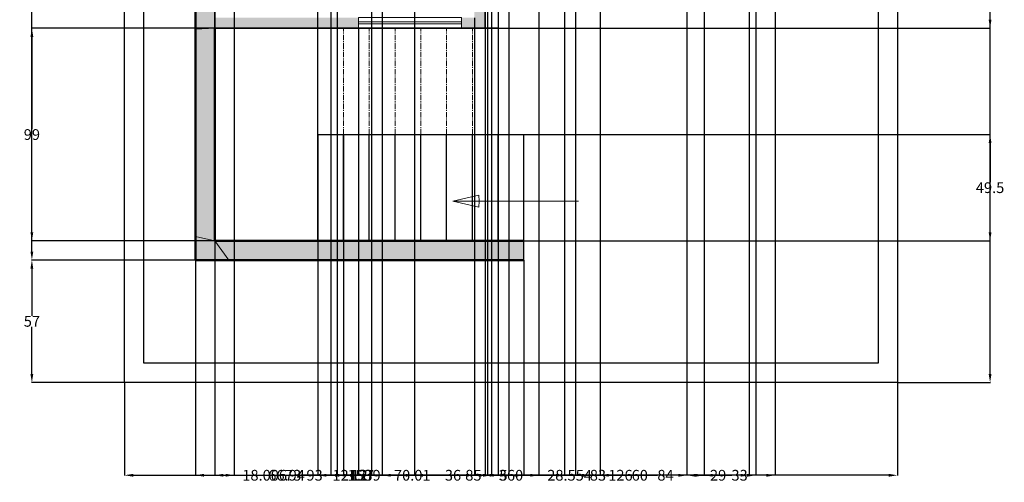
# Model space of a CAD drawing. Units: inches. Extents: x 882 to 1363, y 890 to 1847.
# Tile 1 of 9: x 901 to 1360, y 890 to 1106. Entities that reach past the tile are written whole.
import ezdxf

# ---------------------------------------------------------------- set-up
doc = ezdxf.new("R2010")
doc.units = ezdxf.units.IN
doc.header["$MEASUREMENT"] = 0
doc.linetypes.add('CENTERX2', pattern=[4, 2.5, -0.5, 0.5, -0.5])
for name, color, linetype, lineweight in [('A-ANNO-DIMS', 2, 'Continuous', 18), ('A-ANNO-SYMB', 7, 'Continuous', 18), ('A-FLOR-STRS', 7, 'Continuous', 25), ('A-FLOR-STRS-BYND', 7, 'CENTERX2', 18), ('A-WALL-PATT-BNDY', 7, 'Continuous', 13), ('C-PROP', 7, 'Continuous', 25), ('inner wall', 50, 'Continuous', 35), ('outer wall', 40, 'Continuous', 50), ('windows', 226, 'Continuous', 18)]:
    doc.layers.add(name, color=color, linetype=linetype, lineweight=lineweight)
doc.layers.add('A-WALL-PATT', color=251, linetype='Continuous', lineweight=13, true_color=0x636466)
doc.styles.get("Standard").update_dxf_attribs({"font": 'arial.ttf'})
doc.dimstyles.get("Standard").update_dxf_attribs({"dimtxt": 5, "dimasz": 4, "dimexe": 0.18, "dimexo": 0.0625, "dimgap": 0.09, "dimtad": 0, "dimtih": 1, "dimtoh": 1, "dimdec": 1, "dimzin": 0, "dimdsep": 46, "dimlunit": 3, "dimtxsty": 'Standard', "dimcen": 0.09, "dimadec": 0, "dimazin": 0, "dimtfac": 1, "dimtdec": 1, "dimtofl": 0, "dimtmove": 0, "dimatfit": 3, "dimfxl": 1, "dimtolj": 1, "dimtzin": 0, "dimarcsym": 0})

# ---------------------------------------------------------------- blocks, each defined once
blk = doc.blocks.new('*D33')
at = {"layer": 'A-ANNO-DIMS', "color": 0, "lineweight": -2, "transparency": 16777216}
for p, q in [((949.84, 936.69), (949.84, 893.37)), ((1309.84, 936.69), (1309.84, 893.37)), ((953.84, 893.55), (1124.24, 893.55)), ((1305.84, 893.55), (1135.44, 893.55))]:
    blk.add_line(p, q, dxfattribs=at)
at = {"layer": 'A-ANNO-DIMS', "color": 0, "transparency": 16777216}
for points in [[(953.84, 894.21), (953.84, 892.88), (949.84, 893.55)], [(1305.84, 894.21), (1305.84, 892.88), (1309.84, 893.55)]]:
    blk.add_solid(points, dxfattribs=at)
at = {"layer": 'Defpoints', "color": 0, "transparency": 16777216}
for p in [(949.84, 936.75), (1309.84, 936.75), (1309.84, 893.55)]:
    blk.add_point(p, dxfattribs=at)
at = {"layer": 'A-ANNO-DIMS', "color": 0, "transparency": 16777216, "insert": (1129.84, 893.55), "char_height": 5, "attachment_point": 5}
blk.add_mtext('\\A1;360', dxfattribs=at)
blk = doc.blocks.new('*D34')
at = {"layer": 'A-ANNO-DIMS', "color": 0, "lineweight": -2, "transparency": 16777216}
for p, q in [((1309.9, 1800.75), (1353.22, 1800.75)), ((1353.04, 1796.75), (1353.04, 1371.39)), ((1353.04, 940.75), (1353.04, 1366.11)), ((1309.9, 936.75), (1353.22, 936.75))]:
    blk.add_line(p, q, dxfattribs=at)
at = {"layer": 'A-ANNO-DIMS', "color": 0, "transparency": 16777216}
for points in [[(1352.38, 1796.75), (1353.71, 1796.75), (1353.04, 1800.75)], [(1352.38, 940.75), (1353.71, 940.75), (1353.04, 936.75)]]:
    blk.add_solid(points, dxfattribs=at)
at = {"layer": 'Defpoints', "color": 0, "transparency": 16777216}
for p in [(1309.84, 1800.75), (1353.04, 1800.75), (1309.84, 936.75)]:
    blk.add_point(p, dxfattribs=at)
at = {"layer": 'A-ANNO-DIMS', "color": 0, "transparency": 16777216, "insert": (1353.04, 1368.75), "char_height": 5, "attachment_point": 5}
blk.add_mtext('\\A1;864', dxfattribs=at)
blk = doc.blocks.new('*D36')
at = {"layer": 'A-ANNO-DIMS', "color": 0, "lineweight": -2, "transparency": 16777216}
for p, q in [((982.78, 993.75), (906.46, 993.75)), ((906.64, 989.75), (906.64, 967.88)), ((906.64, 940.75), (906.64, 962.62)), ((949.78, 936.75), (906.46, 936.75))]:
    blk.add_line(p, q, dxfattribs=at)
at = {"layer": 'A-ANNO-DIMS', "color": 0, "transparency": 16777216}
for points in [[(905.97, 989.75), (907.3, 989.75), (906.64, 993.75)], [(905.97, 940.75), (907.3, 940.75), (906.64, 936.75)]]:
    blk.add_solid(points, dxfattribs=at)
at = {"layer": 'Defpoints', "color": 0, "transparency": 16777216}
for p in [(906.64, 993.75), (982.84, 993.75), (949.84, 936.75)]:
    blk.add_point(p, dxfattribs=at)
at = {"layer": 'A-ANNO-DIMS', "color": 0, "transparency": 16777216, "insert": (906.64, 965.25), "char_height": 5, "attachment_point": 5}
blk.add_mtext('\\A1;57', dxfattribs=at)
blk = doc.blocks.new('*D37')
at = {"layer": 'A-ANNO-DIMS', "color": 0, "lineweight": -2, "transparency": 16777216}
for p, q in [((982.78, 1767.75), (906.46, 1767.75)), ((906.64, 1763.75), (906.64, 1383.34)), ((906.64, 997.75), (906.64, 1378.16)), ((982.78, 993.75), (906.46, 993.75))]:
    blk.add_line(p, q, dxfattribs=at)
at = {"layer": 'A-ANNO-DIMS', "color": 0, "transparency": 16777216}
for points in [[(905.97, 1763.75), (907.3, 1763.75), (906.64, 1767.75)], [(905.97, 997.75), (907.3, 997.75), (906.64, 993.75)]]:
    blk.add_solid(points, dxfattribs=at)
at = {"layer": 'Defpoints', "color": 0, "transparency": 16777216}
for p in [(906.64, 1767.75), (982.84, 1767.75), (982.84, 993.75)]:
    blk.add_point(p, dxfattribs=at)
at = {"layer": 'A-ANNO-DIMS', "color": 0, "transparency": 16777216, "insert": (906.64, 1380.75), "char_height": 5, "attachment_point": 5}
blk.add_mtext('\\A1;774', dxfattribs=at)
blk = doc.blocks.new('*D40')
at = {"layer": 'A-ANNO-DIMS', "color": 0, "lineweight": -2, "transparency": 16777216}
for p, q in [((991.84, 1758.69), (991.84, 893.37)), ((1064.84, 1758.69), (1064.84, 893.37)), ((995.84, 893.55), (1024.69, 893.55)), ((1060.84, 893.55), (1031.99, 893.55))]:
    blk.add_line(p, q, dxfattribs=at)
at = {"layer": 'A-ANNO-DIMS', "color": 0, "transparency": 16777216}
for points in [[(995.84, 894.21), (995.84, 892.88), (991.84, 893.55)], [(1060.84, 894.21), (1060.84, 892.88), (1064.84, 893.55)]]:
    blk.add_solid(points, dxfattribs=at)
at = {"layer": 'Defpoints', "color": 0, "transparency": 16777216}
for p in [(991.84, 1758.75), (1064.84, 1758.75), (1064.84, 893.55)]:
    blk.add_point(p, dxfattribs=at)
at = {"layer": 'A-ANNO-DIMS', "color": 0, "transparency": 16777216, "insert": (1028.34, 893.55), "char_height": 5, "attachment_point": 5}
blk.add_mtext('\\A1;73', dxfattribs=at)
blk = doc.blocks.new('*D41')
at = {"layer": 'A-ANNO-DIMS', "color": 0, "lineweight": -2, "transparency": 16777216}
for p, q in [((1069.84, 1758.69), (1069.84, 893.37)), ((1154.84, 1758.69), (1154.84, 893.37)), ((1073.84, 893.55), (1108.65, 893.55)), ((1150.84, 893.55), (1116.03, 893.55))]:
    blk.add_line(p, q, dxfattribs=at)
at = {"layer": 'A-ANNO-DIMS', "color": 0, "transparency": 16777216}
for points in [[(1073.84, 894.21), (1073.84, 892.88), (1069.84, 893.55)], [(1150.84, 894.21), (1150.84, 892.88), (1154.84, 893.55)]]:
    blk.add_solid(points, dxfattribs=at)
at = {"layer": 'Defpoints', "color": 0, "transparency": 16777216}
for p in [(1069.84, 1758.75), (1154.84, 1758.75), (1154.84, 893.55)]:
    blk.add_point(p, dxfattribs=at)
at = {"layer": 'A-ANNO-DIMS', "color": 0, "transparency": 16777216, "insert": (1112.34, 893.55), "char_height": 5, "attachment_point": 5}
blk.add_mtext('\\A1;85', dxfattribs=at)
blk = doc.blocks.new('*D42')
at = {"layer": 'A-ANNO-DIMS', "color": 0, "lineweight": -2, "transparency": 16777216}
for p, q in [((1159.84, 1710.69), (1159.84, 893.37)), ((1243.84, 1705.69), (1243.84, 893.37)), ((1163.84, 893.55), (1198.17, 893.55)), ((1239.84, 893.55), (1205.5, 893.55))]:
    blk.add_line(p, q, dxfattribs=at)
at = {"layer": 'A-ANNO-DIMS', "color": 0, "transparency": 16777216}
for points in [[(1163.84, 894.21), (1163.84, 892.88), (1159.84, 893.55)], [(1239.84, 894.21), (1239.84, 892.88), (1243.84, 893.55)]]:
    blk.add_solid(points, dxfattribs=at)
at = {"layer": 'Defpoints', "color": 0, "transparency": 16777216}
for p in [(1159.84, 1710.75), (1243.84, 1705.75), (1243.84, 893.55)]:
    blk.add_point(p, dxfattribs=at)
at = {"layer": 'A-ANNO-DIMS', "color": 0, "transparency": 16777216, "insert": (1201.84, 893.55), "char_height": 5, "attachment_point": 5}
blk.add_mtext('\\A1;84', dxfattribs=at)
blk = doc.blocks.new('*D47')
at = {"layer": 'A-ANNO-DIMS', "color": 0, "lineweight": -2, "transparency": 16777216}
for p, q in [((1123.84, 1567.69), (1123.84, 893.37)), ((1128.84, 1567.69), (1128.84, 893.37)), ((1119.84, 893.55), (1115.84, 893.55)), ((1132.84, 893.55), (1136.84, 893.55))]:
    blk.add_line(p, q, dxfattribs=at)
at = {"layer": 'A-ANNO-DIMS', "color": 0, "transparency": 16777216}
for points in [[(1119.84, 894.21), (1119.84, 892.88), (1123.84, 893.55)], [(1132.84, 894.21), (1132.84, 892.88), (1128.84, 893.55)]]:
    blk.add_solid(points, dxfattribs=at)
at = {"layer": 'Defpoints', "color": 0, "transparency": 16777216}
for p in [(1123.84, 1567.75), (1128.84, 1567.75), (1128.84, 893.55)]:
    blk.add_point(p, dxfattribs=at)
at = {"layer": 'A-ANNO-DIMS', "color": 0, "transparency": 16777216, "insert": (1126.34, 893.55), "char_height": 5, "attachment_point": 5}
blk.add_mtext('\\A1;5', dxfattribs=at)
blk = doc.blocks.new('*D48')
at = {"layer": 'A-ANNO-DIMS', "color": 0, "lineweight": -2, "transparency": 16777216}
for p, q in [((1084.84, 1562.69), (1084.84, 893.37)), ((1120.84, 1562.69), (1120.84, 893.37)), ((1088.84, 893.55), (1099.17, 893.55)), ((1116.84, 893.55), (1106.51, 893.55))]:
    blk.add_line(p, q, dxfattribs=at)
at = {"layer": 'A-ANNO-DIMS', "color": 0, "transparency": 16777216}
for points in [[(1088.84, 894.21), (1088.84, 892.88), (1084.84, 893.55)], [(1116.84, 894.21), (1116.84, 892.88), (1120.84, 893.55)]]:
    blk.add_solid(points, dxfattribs=at)
at = {"layer": 'Defpoints', "color": 0, "transparency": 16777216}
for p in [(1084.84, 1562.75), (1120.84, 1562.75), (1120.84, 893.55)]:
    blk.add_point(p, dxfattribs=at)
at = {"layer": 'A-ANNO-DIMS', "color": 0, "transparency": 16777216, "insert": (1102.84, 893.55), "char_height": 5, "attachment_point": 5}
blk.add_mtext('\\A1;36', dxfattribs=at)
blk = doc.blocks.new('*D49')
at = {"layer": 'A-ANNO-DIMS', "color": 0, "lineweight": -2, "transparency": 16777216}
for p, q in [((1211.84, 1562.69), (1211.84, 893.37)), ((1240.84, 1562.69), (1240.84, 893.37)), ((1215.84, 893.55), (1222.62, 893.55)), ((1236.84, 893.55), (1230.06, 893.55))]:
    blk.add_line(p, q, dxfattribs=at)
at = {"layer": 'A-ANNO-DIMS', "color": 0, "transparency": 16777216}
for points in [[(1215.84, 894.21), (1215.84, 892.88), (1211.84, 893.55)], [(1236.84, 894.21), (1236.84, 892.88), (1240.84, 893.55)]]:
    blk.add_solid(points, dxfattribs=at)
at = {"layer": 'Defpoints', "color": 0, "transparency": 16777216}
for p in [(1211.84, 1562.75), (1240.84, 1562.75), (1240.84, 893.55)]:
    blk.add_point(p, dxfattribs=at)
at = {"layer": 'A-ANNO-DIMS', "color": 0, "transparency": 16777216, "insert": (1226.34, 893.55), "char_height": 5, "attachment_point": 5}
blk.add_mtext('\\A1;29', dxfattribs=at)
blk = doc.blocks.new('*D51')
at = {"layer": 'A-ANNO-DIMS', "color": 0, "lineweight": -2, "transparency": 16777216}
for p, q in [((982.84, 1767.69), (982.84, 893.37)), ((1000.84, 1767.69), (1000.84, 893.37)), ((986.84, 893.55), (996.84, 893.55)), ((1000.84, 893.55), (1004.84, 893.55))]:
    blk.add_line(p, q, dxfattribs=at)
at = {"layer": 'A-ANNO-DIMS', "color": 0, "transparency": 16777216}
for points in [[(986.84, 894.21), (986.84, 892.88), (982.84, 893.55)], [(996.84, 894.21), (996.84, 892.88), (1000.84, 893.55)]]:
    blk.add_solid(points, dxfattribs=at)
at = {"layer": 'Defpoints', "color": 0, "transparency": 16777216}
for p in [(982.84, 1767.75), (1000.84, 1767.75), (1000.84, 893.55)]:
    blk.add_point(p, dxfattribs=at)
at = {"layer": 'A-ANNO-DIMS', "color": 0, "transparency": 16777216, "insert": (1015.08, 893.55), "char_height": 5, "attachment_point": 5}
blk.add_mtext('\\A1;18.006', dxfattribs=at)
blk = doc.blocks.new('*D52')
at = {"layer": 'A-ANNO-DIMS', "color": 0, "lineweight": -2, "transparency": 16777216}
for p, q in [((1048.84, 1767.69), (1048.84, 893.37)), ((1118.86, 1767.69), (1118.86, 893.37)), ((1052.84, 893.55), (1075.83, 893.55)), ((1114.86, 893.55), (1091.87, 893.55))]:
    blk.add_line(p, q, dxfattribs=at)
at = {"layer": 'A-ANNO-DIMS', "color": 0, "transparency": 16777216}
for points in [[(1052.84, 894.21), (1052.84, 892.88), (1048.84, 893.55)], [(1114.86, 894.21), (1114.86, 892.88), (1118.86, 893.55)]]:
    blk.add_solid(points, dxfattribs=at)
at = {"layer": 'Defpoints', "color": 0, "transparency": 16777216}
for p in [(1048.84, 1767.75), (1118.86, 1767.75), (1118.86, 893.55)]:
    blk.add_point(p, dxfattribs=at)
at = {"layer": 'A-ANNO-DIMS', "color": 0, "transparency": 16777216, "insert": (1083.85, 893.55), "char_height": 5, "attachment_point": 5}
blk.add_mtext('\\A1;70.01', dxfattribs=at)
blk = doc.blocks.new('*D53')
at = {"layer": 'A-ANNO-DIMS', "color": 0, "lineweight": -2, "transparency": 16777216}
for p, q in [((1142.86, 1767.69), (1142.86, 893.37)), ((1171.41, 1767.69), (1171.41, 893.37)), ((1138.86, 893.55), (1134.86, 893.55)), ((1175.41, 893.55), (1179.41, 893.55))]:
    blk.add_line(p, q, dxfattribs=at)
at = {"layer": 'A-ANNO-DIMS', "color": 0, "transparency": 16777216}
for points in [[(1138.86, 894.21), (1138.86, 892.88), (1142.86, 893.55)], [(1175.41, 894.21), (1175.41, 892.88), (1171.41, 893.55)]]:
    blk.add_solid(points, dxfattribs=at)
at = {"layer": 'Defpoints', "color": 0, "transparency": 16777216}
for p in [(1142.86, 1767.75), (1171.41, 1767.75), (1171.41, 893.55)]:
    blk.add_point(p, dxfattribs=at)
at = {"layer": 'A-ANNO-DIMS', "color": 0, "transparency": 16777216, "insert": (1157.14, 893.55), "char_height": 5, "attachment_point": 5}
blk.add_mtext('\\A1;28.554', dxfattribs=at)
blk = doc.blocks.new('*D61')
at = {"layer": 'A-ANNO-DIMS', "color": 0, "lineweight": -2, "transparency": 16777216}
for p, q in [((991.84, 1348.69), (991.84, 893.37)), ((1128.84, 1348.69), (1128.84, 893.37)), ((995.84, 893.55), (1054.96, 893.55)), ((1124.84, 893.55), (1065.72, 893.55))]:
    blk.add_line(p, q, dxfattribs=at)
at = {"layer": 'A-ANNO-DIMS', "color": 0, "transparency": 16777216}
for points in [[(995.84, 894.21), (995.84, 892.88), (991.84, 893.55)], [(1124.84, 894.21), (1124.84, 892.88), (1128.84, 893.55)]]:
    blk.add_solid(points, dxfattribs=at)
at = {"layer": 'Defpoints', "color": 0, "transparency": 16777216}
for p in [(991.84, 1348.75), (1128.84, 1348.75), (1128.84, 893.55)]:
    blk.add_point(p, dxfattribs=at)
at = {"layer": 'A-ANNO-DIMS', "color": 0, "transparency": 16777216, "insert": (1060.34, 893.55), "char_height": 5, "attachment_point": 5}
blk.add_mtext('\\A1;137', dxfattribs=at)
blk = doc.blocks.new('*D63')
at = {"layer": 'A-ANNO-DIMS', "color": 0, "lineweight": -2, "transparency": 16777216}
for p, q in [((991.84, 1106.69), (991.84, 893.37)), ((1112.84, 1106.69), (1112.84, 893.37)), ((995.84, 893.55), (1047.44, 893.55)), ((1108.84, 893.55), (1057.23, 893.55))]:
    blk.add_line(p, q, dxfattribs=at)
at = {"layer": 'A-ANNO-DIMS', "color": 0, "transparency": 16777216}
for points in [[(995.84, 894.21), (995.84, 892.88), (991.84, 893.55)], [(1108.84, 894.21), (1108.84, 892.88), (1112.84, 893.55)]]:
    blk.add_solid(points, dxfattribs=at)
at = {"layer": 'Defpoints', "color": 0, "transparency": 16777216}
for p in [(991.84, 1106.75), (1112.84, 1106.75), (1112.84, 893.55)]:
    blk.add_point(p, dxfattribs=at)
at = {"layer": 'A-ANNO-DIMS', "color": 0, "transparency": 16777216, "insert": (1052.34, 893.55), "char_height": 5, "attachment_point": 5}
blk.add_mtext('\\A1;121', dxfattribs=at)
blk = doc.blocks.new('*D64')
at = {"layer": 'A-ANNO-DIMS', "color": 0, "lineweight": -2, "transparency": 16777216}
for p, q in [((1117.84, 1269.69), (1117.84, 893.37)), ((1243.84, 1269.69), (1243.84, 893.37)), ((1121.84, 893.55), (1175.46, 893.55)), ((1239.84, 893.55), (1186.22, 893.55))]:
    blk.add_line(p, q, dxfattribs=at)
at = {"layer": 'A-ANNO-DIMS', "color": 0, "transparency": 16777216}
for points in [[(1121.84, 894.21), (1121.84, 892.88), (1117.84, 893.55)], [(1239.84, 894.21), (1239.84, 892.88), (1243.84, 893.55)]]:
    blk.add_solid(points, dxfattribs=at)
at = {"layer": 'Defpoints', "color": 0, "transparency": 16777216}
for p in [(1117.84, 1269.75), (1243.84, 1269.75), (1243.84, 893.55)]:
    blk.add_point(p, dxfattribs=at)
at = {"layer": 'A-ANNO-DIMS', "color": 0, "transparency": 16777216, "insert": (1180.84, 893.55), "char_height": 5, "attachment_point": 5}
blk.add_mtext('\\A1;126', dxfattribs=at)
blk = doc.blocks.new('*D66')
at = {"layer": 'A-ANNO-DIMS', "color": 0, "lineweight": -2, "transparency": 16777216}
for p, q in [((1159.84, 1144.69), (1159.84, 893.37)), ((1219.84, 1144.69), (1219.84, 893.37)), ((1163.84, 893.55), (1186.16, 893.55)), ((1215.84, 893.55), (1193.52, 893.55))]:
    blk.add_line(p, q, dxfattribs=at)
at = {"layer": 'A-ANNO-DIMS', "color": 0, "transparency": 16777216}
for points in [[(1163.84, 894.21), (1163.84, 892.88), (1159.84, 893.55)], [(1215.84, 894.21), (1215.84, 892.88), (1219.84, 893.55)]]:
    blk.add_solid(points, dxfattribs=at)
at = {"layer": 'Defpoints', "color": 0, "transparency": 16777216}
for p in [(1159.84, 1144.75), (1219.84, 1144.75), (1219.84, 893.55)]:
    blk.add_point(p, dxfattribs=at)
at = {"layer": 'A-ANNO-DIMS', "color": 0, "transparency": 16777216, "insert": (1189.84, 893.55), "char_height": 5, "attachment_point": 5}
blk.add_mtext('\\A1;60', dxfattribs=at)
blk = doc.blocks.new('*D72')
at = {"layer": 'A-ANNO-DIMS', "color": 0, "lineweight": -2, "transparency": 16777216}
for p, q in [((982.84, 993.69), (982.84, 893.37)), ((1135.84, 993.69), (1135.84, 893.37)), ((986.84, 893.55), (1053.96, 893.55)), ((1131.84, 893.55), (1064.72, 893.55))]:
    blk.add_line(p, q, dxfattribs=at)
at = {"layer": 'A-ANNO-DIMS', "color": 0, "transparency": 16777216}
for points in [[(986.84, 894.21), (986.84, 892.88), (982.84, 893.55)], [(1131.84, 894.21), (1131.84, 892.88), (1135.84, 893.55)]]:
    blk.add_solid(points, dxfattribs=at)
at = {"layer": 'Defpoints', "color": 0, "transparency": 16777216}
for p in [(982.84, 993.75), (1135.84, 993.75), (1135.84, 893.55)]:
    blk.add_point(p, dxfattribs=at)
at = {"layer": 'A-ANNO-DIMS', "color": 0, "transparency": 16777216, "insert": (1059.34, 893.55), "char_height": 5, "attachment_point": 5}
blk.add_mtext('\\A1;153', dxfattribs=at)
blk = doc.blocks.new('*D73')
at = {"layer": 'A-ANNO-DIMS', "color": 0, "lineweight": -2, "transparency": 16777216}
for p, q in [((991.78, 1101.75), (906.46, 1101.75)), ((906.64, 1097.75), (906.64, 1054.89)), ((906.64, 1006.75), (906.64, 1049.61)), ((991.78, 1002.75), (906.46, 1002.75))]:
    blk.add_line(p, q, dxfattribs=at)
at = {"layer": 'A-ANNO-DIMS', "color": 0, "transparency": 16777216}
for points in [[(905.97, 1097.75), (907.3, 1097.75), (906.64, 1101.75)], [(905.97, 1006.75), (907.3, 1006.75), (906.64, 1002.75)]]:
    blk.add_solid(points, dxfattribs=at)
at = {"layer": 'Defpoints', "color": 0, "transparency": 16777216}
for p in [(906.64, 1101.75), (991.84, 1101.75), (991.84, 1002.75)]:
    blk.add_point(p, dxfattribs=at)
at = {"layer": 'A-ANNO-DIMS', "color": 0, "transparency": 16777216, "insert": (906.64, 1052.25), "char_height": 5, "attachment_point": 5}
blk.add_mtext('\\A1;99', dxfattribs=at)
blk = doc.blocks.new('*D74')
at = {"layer": 'A-ANNO-DIMS', "color": 0, "lineweight": -2, "transparency": 16777216}
for p, q in [((991.84, 1002.81), (991.84, 1844.13)), ((1039.84, 1002.81), (1039.84, 1844.13)), ((995.84, 1843.95), (1012.06, 1843.95)), ((1035.84, 1843.95), (1019.62, 1843.95))]:
    blk.add_line(p, q, dxfattribs=at)
at = {"layer": 'A-ANNO-DIMS', "color": 0, "transparency": 16777216}
for points in [[(995.84, 1844.62), (995.84, 1843.29), (991.84, 1843.95)], [(1035.84, 1844.62), (1035.84, 1843.29), (1039.84, 1843.95)]]:
    blk.add_solid(points, dxfattribs=at)
at = {"layer": 'Defpoints', "color": 0, "transparency": 16777216}
for p in [(1039.84, 1843.95), (991.84, 1002.75), (1039.84, 1002.75)]:
    blk.add_point(p, dxfattribs=at)
at = {"layer": 'A-ANNO-DIMS', "color": 0, "transparency": 16777216, "insert": (1015.84, 1843.95), "char_height": 5, "attachment_point": 5}
blk.add_mtext('\\A1;48', dxfattribs=at)
blk = doc.blocks.new('*D75')
at = {"layer": 'A-ANNO-DIMS', "color": 0, "lineweight": -2, "transparency": 16777216}
for p, q in [((1039.84, 1052.19), (1039.84, 893.37)), ((1051.84, 1052.19), (1051.84, 893.37)), ((1043.84, 893.55), (1047.84, 893.55)), ((1051.84, 893.55), (1055.84, 893.55))]:
    blk.add_line(p, q, dxfattribs=at)
at = {"layer": 'A-ANNO-DIMS', "color": 0, "transparency": 16777216}
for points in [[(1043.84, 894.21), (1043.84, 892.88), (1039.84, 893.55)], [(1047.84, 894.21), (1047.84, 892.88), (1051.84, 893.55)]]:
    blk.add_solid(points, dxfattribs=at)
at = {"layer": 'Defpoints', "color": 0, "transparency": 16777216}
for p in [(1039.84, 1052.25), (1051.84, 1052.25), (1051.84, 893.55)]:
    blk.add_point(p, dxfattribs=at)
at = {"layer": 'A-ANNO-DIMS', "color": 0, "transparency": 16777216, "insert": (1059.25, 893.55), "char_height": 5, "attachment_point": 5}
blk.add_mtext('\\A1;12', dxfattribs=at)
blk = doc.blocks.new('*D76')
at = {"layer": 'A-ANNO-DIMS', "color": 0, "lineweight": -2, "transparency": 16777216}
for p, q in [((1135.9, 1052.25), (1353.22, 1052.25)), ((1353.04, 1048.25), (1353.04, 1030.14)), ((1353.04, 1006.75), (1353.04, 1024.86)), ((1135.9, 1002.75), (1353.22, 1002.75))]:
    blk.add_line(p, q, dxfattribs=at)
at = {"layer": 'A-ANNO-DIMS', "color": 0, "transparency": 16777216}
for points in [[(1352.38, 1048.25), (1353.71, 1048.25), (1353.04, 1052.25)], [(1352.38, 1006.75), (1353.71, 1006.75), (1353.04, 1002.75)]]:
    blk.add_solid(points, dxfattribs=at)
at = {"layer": 'Defpoints', "color": 0, "transparency": 16777216}
for p in [(1135.84, 1052.25), (1353.04, 1052.25), (1135.84, 1002.75)]:
    blk.add_point(p, dxfattribs=at)
at = {"layer": 'A-ANNO-DIMS', "color": 0, "transparency": 16777216, "insert": (1353.04, 1027.5), "char_height": 5, "attachment_point": 5}
blk.add_mtext('\\A1;49.5', dxfattribs=at)
blk = doc.blocks.new('*D77')
at = {"layer": 'A-ANNO-DIMS', "color": 0, "lineweight": -2, "transparency": 16777216}
for p, q in [((1117.9, 1144.75), (1353.22, 1144.75)), ((1353.04, 1140.75), (1353.04, 1125.89)), ((1353.04, 1105.75), (1353.04, 1120.6)), ((1117.9, 1101.75), (1353.22, 1101.75))]:
    blk.add_line(p, q, dxfattribs=at)
at = {"layer": 'A-ANNO-DIMS', "color": 0, "transparency": 16777216}
for points in [[(1352.38, 1140.75), (1353.71, 1140.75), (1353.04, 1144.75)], [(1352.38, 1105.75), (1353.71, 1105.75), (1353.04, 1101.75)]]:
    blk.add_solid(points, dxfattribs=at)
at = {"layer": 'Defpoints', "color": 0, "transparency": 16777216}
for p in [(1117.84, 1144.75), (1353.04, 1144.75), (1117.84, 1101.75)]:
    blk.add_point(p, dxfattribs=at)
at = {"layer": 'A-ANNO-DIMS', "color": 0, "transparency": 16777216, "insert": (1353.04, 1123.25), "char_height": 5, "attachment_point": 5}
blk.add_mtext('\\A1;43', dxfattribs=at)
blk = doc.blocks.new('*D82')
at = {"layer": 'A-ANNO-DIMS', "color": 0, "lineweight": -2, "transparency": 16777216}
for p, q in [((1219.84, 1144.69), (1219.84, 893.37)), ((1252.84, 1144.69), (1252.84, 893.37)), ((1223.84, 893.55), (1232.67, 893.55)), ((1248.84, 893.55), (1240.01, 893.55))]:
    blk.add_line(p, q, dxfattribs=at)
at = {"layer": 'A-ANNO-DIMS', "color": 0, "transparency": 16777216}
for points in [[(1223.84, 894.21), (1223.84, 892.88), (1219.84, 893.55)], [(1248.84, 894.21), (1248.84, 892.88), (1252.84, 893.55)]]:
    blk.add_solid(points, dxfattribs=at)
at = {"layer": 'Defpoints', "color": 0, "transparency": 16777216}
for p in [(1219.84, 1144.75), (1252.84, 1144.75), (1252.84, 893.55)]:
    blk.add_point(p, dxfattribs=at)
at = {"layer": 'A-ANNO-DIMS', "color": 0, "transparency": 16777216, "insert": (1236.34, 893.55), "char_height": 5, "attachment_point": 5}
blk.add_mtext('\\A1;33', dxfattribs=at)
blk = doc.blocks.new('*D84')
at = {"layer": 'A-ANNO-DIMS', "color": 0, "lineweight": -2, "transparency": 16777216}
for p, q in [((991.84, 1101.69), (991.84, 893.37)), ((1058.78, 1101.69), (1058.78, 893.37)), ((995.84, 893.55), (1016.78, 893.55)), ((1054.78, 893.55), (1033.84, 893.55))]:
    blk.add_line(p, q, dxfattribs=at)
at = {"layer": 'A-ANNO-DIMS', "color": 0, "transparency": 16777216}
for points in [[(995.84, 894.21), (995.84, 892.88), (991.84, 893.55)], [(1054.78, 894.21), (1054.78, 892.88), (1058.78, 893.55)]]:
    blk.add_solid(points, dxfattribs=at)
at = {"layer": 'Defpoints', "color": 0, "transparency": 16777216}
for p in [(991.84, 1101.75), (1058.78, 1101.75), (1058.78, 893.55)]:
    blk.add_point(p, dxfattribs=at)
at = {"layer": 'A-ANNO-DIMS', "color": 0, "transparency": 16777216, "insert": (1025.31, 893.55), "char_height": 5, "attachment_point": 5}
blk.add_mtext('\\A1;66.94', dxfattribs=at)
blk = doc.blocks.new('*D85')
at = {"layer": 'A-ANNO-DIMS', "color": 0, "lineweight": -2, "transparency": 16777216}
for p, q in [((1045.84, 1562.69), (1045.84, 893.37)), ((1084.84, 1562.69), (1084.84, 893.37)), ((1049.84, 893.55), (1061.66, 893.55)), ((1080.84, 893.55), (1069.01, 893.55))]:
    blk.add_line(p, q, dxfattribs=at)
at = {"layer": 'A-ANNO-DIMS', "color": 0, "transparency": 16777216}
for points in [[(1049.84, 894.21), (1049.84, 892.88), (1045.84, 893.55)], [(1080.84, 894.21), (1080.84, 892.88), (1084.84, 893.55)]]:
    blk.add_solid(points, dxfattribs=at)
at = {"layer": 'Defpoints', "color": 0, "transparency": 16777216}
for p in [(1045.84, 1562.75), (1084.84, 1562.75), (1084.84, 893.55)]:
    blk.add_point(p, dxfattribs=at)
at = {"layer": 'A-ANNO-DIMS', "color": 0, "transparency": 16777216, "insert": (1065.34, 893.55), "char_height": 5, "attachment_point": 5}
blk.add_mtext('\\A1;39', dxfattribs=at)
blk = doc.blocks.new('*D88')
at = {"layer": 'A-ANNO-DIMS', "color": 0, "lineweight": -2, "transparency": 16777216}
for p, q in [((1128.84, 1567.69), (1128.84, 893.37)), ((1211.84, 1562.69), (1211.84, 893.37)), ((1132.84, 893.55), (1166.66, 893.55)), ((1207.84, 893.55), (1174.01, 893.55))]:
    blk.add_line(p, q, dxfattribs=at)
at = {"layer": 'A-ANNO-DIMS', "color": 0, "transparency": 16777216}
for points in [[(1132.84, 894.21), (1132.84, 892.88), (1128.84, 893.55)], [(1207.84, 894.21), (1207.84, 892.88), (1211.84, 893.55)]]:
    blk.add_solid(points, dxfattribs=at)
at = {"layer": 'Defpoints', "color": 0, "transparency": 16777216}
for p in [(1128.84, 1567.75), (1211.84, 1562.75), (1211.84, 893.55)]:
    blk.add_point(p, dxfattribs=at)
at = {"layer": 'A-ANNO-DIMS', "color": 0, "transparency": 16777216, "insert": (1170.34, 893.55), "char_height": 5, "attachment_point": 5}
blk.add_mtext('\\A1;83', dxfattribs=at)
blk = doc.blocks.new('*D89')
at = {"layer": 'A-ANNO-DIMS', "color": 0, "lineweight": -2, "transparency": 16777216}
for p, q in [((991.84, 1473.69), (991.84, 893.37)), ((1084.84, 1473.69), (1084.84, 893.37)), ((995.84, 893.55), (1034.67, 893.55)), ((1080.84, 893.55), (1042.01, 893.55))]:
    blk.add_line(p, q, dxfattribs=at)
at = {"layer": 'A-ANNO-DIMS', "color": 0, "transparency": 16777216}
for points in [[(995.84, 894.21), (995.84, 892.88), (991.84, 893.55)], [(1080.84, 894.21), (1080.84, 892.88), (1084.84, 893.55)]]:
    blk.add_solid(points, dxfattribs=at)
at = {"layer": 'Defpoints', "color": 0, "transparency": 16777216}
for p in [(991.84, 1473.75), (1084.84, 1473.75), (1084.84, 893.55)]:
    blk.add_point(p, dxfattribs=at)
at = {"layer": 'A-ANNO-DIMS', "color": 0, "transparency": 16777216, "insert": (1038.34, 893.55), "char_height": 5, "attachment_point": 5}
blk.add_mtext('\\A1;93', dxfattribs=at)

msp = doc.modelspace()

# ---------------------------------------------------------------- hatches: boundary and pattern name
at = {"layer": 'A-WALL-PATT'}
h = msp.add_hatch(color=256, dxfattribs=at)
h.dxf.hatch_style = 1
h.paths.add_polyline_path([(1050.8388, 1481.7495), (1050.8388, 1478.7495), (1084.8388, 1478.7495), (1084.8388, 1473.7495), (991.8388, 1473.7495), (991.8388, 1361.0778), (982.8388, 1361.0778), (982.8388, 1556.1531), (991.8388, 1556.1531), (991.8388, 1478.7495), (1045.8388, 1478.7495), (1045.8388, 1481.7479), (1045.4161, 1481.7477), (1030.9055, 1506.8563), (1032.004, 1507.4911), (1046.5146, 1482.3825), (1045.4161, 1481.7477), (1045.8388, 1481.7479), (1045.8388, 1481.7495)])
h.paths.add_polyline_path([(1128.8388, 1478.7495), (1120.8388, 1478.7495), (1120.8388, 1473.7495), (1123.8388, 1473.7495), (1123.8388, 1353.7495), (991.8388, 1353.7495), (991.8388, 1361.0778), (982.8388, 1361.0778), (982.8388, 1337.3333), (991.8388, 1337.3333), (991.8388, 1348.7495), (1128.8388, 1348.7495)])
h.paths.add_polyline_path([(1118.8585, 1767.7495), (1048.8447, 1767.7495), (1048.8447, 1758.7495), (1064.8388, 1758.7495), (1069.8388, 1758.7495), (1118.8585, 1758.7495)])
h.paths.add_polyline_path([(1171.4129, 1767.7495), (1142.8585, 1767.7495), (1142.8585, 1758.7495), (1154.8388, 1758.7495), (1154.8388, 1710.7495), (1069.8388, 1710.7495), (1069.8388, 1713.7495), (1064.8388, 1713.7495), (1064.8388, 1705.7495), (1123.8388, 1705.7495), (1123.8388, 1567.7495), (1120.8388, 1567.7495), (1120.8388, 1562.7495), (1123.8388, 1562.7495), (1211.8388, 1562.7495), (1211.8388, 1567.7495), (1128.8388, 1567.7495), (1128.8388, 1705.7495), (1211.8388, 1705.7495), (1211.8388, 1710.7495), (1159.8388, 1710.7495), (1159.8388, 1758.7495), (1171.4129, 1758.7495)])
h.paths.add_polyline_path([(1252.8388, 1767.7495), (1195.4129, 1767.7495), (1195.4129, 1758.7495), (1243.8388, 1758.7495), (1243.8388, 1710.7495), (1240.8388, 1710.7495), (1240.8388, 1706.4648), (1240.8388, 1705.7495), (1243.8388, 1705.7495), (1243.8388, 1673.1735), (1252.8388, 1673.1735)])
h.paths.add_polyline_path([(1252.8388, 1625.1735), (1243.8388, 1625.1735), (1243.8388, 1567.7495), (1240.8388, 1567.7495), (1240.8388, 1562.7495), (1243.8388, 1562.7495), (1243.8388, 1546.029), (1252.8388, 1546.029)])
h.paths.add_polyline_path([(1252.8388, 1498.029), (1243.8388, 1498.029), (1243.8388, 1391.1399), (1252.8388, 1391.1399)])
h.paths.add_polyline_path([(1252.8388, 1179.8561), (1243.8388, 1179.8561), (1243.8388, 1149.7495), (1219.8388, 1149.7495), (1219.8388, 1145.3111), (1219.8388, 1144.7495), (1252.8388, 1144.7495)])
h.paths.add_polyline_path([(1252.8388, 1277.7495), (1243.8388, 1277.7495), (1243.8388, 1274.7495), (1219.8388, 1274.7495), (1219.8388, 1269.7495), (1243.8388, 1269.7495), (1243.8388, 1227.8561), (1252.8388, 1227.8561)])
h.paths.add_polyline_path([(1252.8388, 1343.1399), (1243.8388, 1343.1399), (1243.8388, 1313.7495), (1248.3388, 1313.7495), (1252.8388, 1313.7495)])
h.paths.add_polyline_path([(1146.8388, 1274.7495), (1112.8388, 1274.7495), (1112.8388, 1106.7495), (1106.7761, 1106.7495), (1106.7761, 1101.7495), (1117.8388, 1101.7495), (1117.8388, 1144.7495), (1159.8388, 1144.7495), (1159.8388, 1149.7495), (1117.8388, 1149.7495), (1117.8388, 1269.7495), (1146.8388, 1269.7495)])
h = msp.add_hatch(color=256, dxfattribs=at)
h.dxf.hatch_style = 1
h.paths.add_polyline_path([(1000.8447, 1767.7495), (993.3979, 1767.7495), (991.8388, 1758.7495), (1000.8447, 1758.7495)])
h.paths.add_polyline_path([(991.8388, 1654.8981), (982.8388, 1654.3544), (982.8388, 1595.0521), (991.8388, 1594.8981)])
h.paths.add_polyline_path([(991.8388, 1594.8981), (982.8388, 1595.0521), (982.8388, 1559.7196), (991.8388, 1562.7495), (991.8388, 1567.7495)])
h.paths.add_polyline_path([(991.8388, 1562.7495), (982.8388, 1559.7196), (982.8388, 1556.1531), (991.8388, 1556.1531)])
h.paths.add_polyline_path([(991.8388, 1289.3333), (982.8388, 1289.3333), (982.8388, 1265.8272), (991.8388, 1265.8272)])
h.paths.add_polyline_path([(1058.7761, 1106.7495), (991.8388, 1106.7495), (982.8388, 1107.8066), (982.8388, 1101.3439), (991.8388, 1101.7495), (1058.7761, 1101.7495)])
h = msp.add_hatch(color=256, dxfattribs=at)
h.dxf.hatch_style = 1
h.paths.add_polyline_path([(991.8388, 1002.7495), (982.8388, 1004.7121), (982.8388, 993.7495), (998.36, 993.7495)])
h.paths.add_polyline_path([(1135.8388, 1002.7495), (991.8388, 1002.7495), (998.36, 993.7495), (1135.8388, 993.7495)])
h.paths.add_polyline_path([(991.8388, 1101.7495), (982.8388, 1101.3439), (982.8388, 1004.7121), (991.8388, 1002.7495)])
h.paths.add_polyline_path([(991.8388, 1191.1097), (982.8388, 1191.1097), (982.8388, 1107.8066), (991.8388, 1106.7495)])
h.paths.add_polyline_path([(991.8388, 1217.8272), (982.8388, 1217.8272), (982.8388, 1191.1097), (991.8388, 1191.1097)])

# ---------------------------------------------------------------- linework, layer by layer
at = {"layer": 'A-ANNO-SYMB'}
for p, q in [((1102.6718, 1021.1924), (1114.8738, 1023.9486)), ((1114.8738, 1023.9486), (1114.9612, 1021.1924)), ((1161.2274, 1021.1924), (1102.6718, 1021.1924)), ((1102.6718, 1021.1924), (1114.8738, 1018.4361)), ((1114.8738, 1018.4361), (1114.9612, 1021.1924))]:
    msp.add_line(p, q, dxfattribs=at)
at = {"layer": 'A-FLOR-STRS'}
for p, q in [((1039.8388, 1002.7495), (1039.8388, 1101.7495)), ((1039.8388, 1052.2495), (1135.8388, 1052.2495)), ((1051.8388, 1002.7495), (1051.8388, 1052.2495)), ((1063.8388, 1002.7495), (1063.8388, 1052.2495)), ((1075.8388, 1002.7495), (1075.8388, 1052.2495)), ((1075.8388, 1002.7495), (1075.8388, 1052.2495)), ((1087.8388, 1002.7495), (1087.8388, 1052.2495)), ((1099.8388, 1002.7495), (1099.8388, 1052.2495)), ((1111.8388, 1002.7495), (1111.8388, 1052.2495)), ((1123.8388, 1002.7495), (1123.8388, 1052.2495)), ((1135.8388, 993.7495), (1135.8388, 1052.2495))]:
    msp.add_line(p, q, dxfattribs=at)
at = {"layer": 'A-FLOR-STRS-BYND'}
for p, q in [((1051.8388, 1052.2495), (1051.8388, 1101.7495)), ((1063.8388, 1052.2495), (1063.8388, 1101.7495)), ((1075.8388, 1052.2495), (1075.8388, 1101.7495)), ((1087.8388, 1052.2495), (1087.8388, 1101.7495)), ((1099.8388, 1052.2495), (1099.8388, 1101.7495)), ((1111.8388, 1052.2495), (1111.8388, 1101.7495)), ((1123.8388, 1052.2495), (1123.8388, 1101.7495))]:
    msp.add_line(p, q, dxfattribs=at)
at = {"layer": 'A-WALL-PATT-BNDY'}
for p, q in [((991.8388, 1101.7495), (982.8388, 1101.3439)), ((991.8388, 1002.7495), (982.8388, 1004.7121)), ((982.8388, 1004.7121), (991.8388, 1002.7495)), ((991.8388, 1002.7495), (998.36, 993.7495))]:
    msp.add_line(p, q, dxfattribs=at)
at = {"layer": 'C-PROP'}
for points in [[(949.8388, 1800.7495), (1309.8388, 1800.7495), (1309.8388, 936.7495), (949.8388, 936.7495)], [(958.8388, 1791.7495), (1300.8388, 1791.7495), (1300.8388, 945.7495), (958.8388, 945.7495)]]:
    msp.add_lwpolyline(points, close=True, dxfattribs=at)
at = {"layer": 'inner wall'}
for p, q in [((1117.8388, 1144.7495), (1117.8388, 1101.7495)), ((991.8388, 1101.7495), (1123.8388, 1101.7495))]:
    msp.add_line(p, q, dxfattribs=at)
at = {"layer": 'outer wall'}
for p, q in [((982.8388, 993.7495), (982.8388, 1767.7495)), ((991.8388, 1002.7495), (991.8388, 1101.7495)), ((1135.8388, 1002.7495), (991.8388, 1002.7495)), ((1135.8388, 993.7495), (982.8388, 993.7495))]:
    msp.add_line(p, q, dxfattribs=at)
at = {"layer": 'windows'}
for p, q in [((1106.7761, 1104.7495), (1058.7761, 1104.7495)), ((1106.7761, 1103.7495), (1058.7761, 1103.7495))]:
    msp.add_line(p, q, dxfattribs=at)
msp.add_lwpolyline([(1058.7761, 1106.7495), (1106.7761, 1106.7495), (1106.7761, 1101.7495), (1058.7761, 1101.7495)], close=True, dxfattribs=at)

# ---------------------------------------------------------------- dimensions: what is measured, and where the dimension line sits
at = {"layer": 'A-ANNO-DIMS'}
for base, p1, p2, override, picture, middle in [((1039.8388, 1843.953), (991.8388, 1002.7495), (1039.8388, 1002.7495), {"dimdec": 0, "dimlfac": 1, "dimrnd": 0, "dimzin": 0, "dimdsep": 46, "dimlunit": 2}, '*D74', (1015.8388, 1843.953)), ((1000.8447, 893.546), (982.8388, 1767.7495), (1000.8447, 1767.7495), {"dimdec": 3, "dimlfac": 1, "dimrnd": 0, "dimzin": 0, "dimdsep": 46, "dimlunit": 2}, '*D51', (1015.0762, 893.546)), ((1118.8585, 893.546), (1048.8447, 1767.7495), (1118.8585, 1767.7495), {"dimdec": 2, "dimlfac": 1, "dimrnd": 0, "dimzin": 0, "dimdsep": 46, "dimlunit": 2}, '*D52', (1083.8516, 893.546)), ((1171.4129, 893.546), (1142.8585, 1767.7495), (1171.4129, 1767.7495), {"dimdec": 3, "dimlfac": 1, "dimrnd": 0, "dimzin": 0, "dimdsep": 46, "dimlunit": 2}, '*D53', (1157.1357, 893.546)), ((1064.8388, 893.546), (991.8388, 1758.7495), (1064.8388, 1758.7495), {"dimdec": 0, "dimlfac": 1, "dimrnd": 0, "dimzin": 0, "dimdsep": 46, "dimlunit": 2}, '*D40', (1028.3388, 893.546)), ((1154.8388, 893.546), (1069.8388, 1758.7495), (1154.8388, 1758.7495), {"dimdec": 0, "dimlfac": 1, "dimrnd": 0, "dimzin": 0, "dimdsep": 46, "dimlunit": 2}, '*D41', (1112.3388, 893.546)), ((1243.8388, 893.546), (1159.8388, 1710.7495), (1243.8388, 1705.7495), {"dimdec": 0, "dimlfac": 1, "dimrnd": 0, "dimzin": 0, "dimdsep": 46, "dimlunit": 2}, '*D42', (1201.8388, 893.546)), ((1128.8388, 893.546), (1123.8388, 1567.7495), (1128.8388, 1567.7495), {"dimdec": 0, "dimlfac": 1, "dimrnd": 0, "dimzin": 0, "dimdsep": 46, "dimlunit": 2}, '*D47', (1126.3388, 893.546)), ((1211.8388, 893.546), (1128.8388, 1567.7495), (1211.8388, 1562.7495), {"dimdec": 0, "dimlfac": 1, "dimrnd": 0, "dimzin": 0, "dimdsep": 46, "dimlunit": 2}, '*D88', (1170.3388, 893.546)), ((1084.8388, 893.546), (1045.8388, 1562.7495), (1084.8388, 1562.7495), {"dimdec": 0, "dimlfac": 1, "dimrnd": 0, "dimzin": 0, "dimdsep": 46, "dimlunit": 2}, '*D85', (1065.3388, 893.546)), ((1120.8388, 893.546), (1084.8388, 1562.7495), (1120.8388, 1562.7495), {"dimdec": 0, "dimlfac": 1, "dimrnd": 0, "dimzin": 0, "dimdsep": 46, "dimlunit": 2}, '*D48', (1102.8388, 893.546)), ((1240.8388, 893.546), (1211.8388, 1562.7495), (1240.8388, 1562.7495), {"dimdec": 0, "dimlfac": 1, "dimrnd": 0, "dimzin": 0, "dimdsep": 46, "dimlunit": 2}, '*D49', (1226.3388, 893.546)), ((1084.8388, 893.546), (991.8388, 1473.7495), (1084.8388, 1473.7495), {"dimdec": 0, "dimlfac": 1, "dimrnd": 0, "dimzin": 0, "dimdsep": 46, "dimlunit": 2}, '*D89', (1038.3388, 893.546)), ((1128.8388, 893.546), (991.8388, 1348.7495), (1128.8388, 1348.7495), {"dimdec": 0, "dimlfac": 1, "dimrnd": 0, "dimzin": 0, "dimdsep": 46, "dimlunit": 2}, '*D61', (1060.3388, 893.546)), ((1243.8388, 893.546), (1117.8388, 1269.7495), (1243.8388, 1269.7495), {"dimdec": 0, "dimlfac": 1, "dimrnd": 0, "dimzin": 0, "dimdsep": 46, "dimlunit": 2}, '*D64', (1180.8388, 893.546)), ((1219.8388, 893.546), (1159.8388, 1144.7495), (1219.8388, 1144.7495), {"dimdec": 0, "dimlfac": 1, "dimrnd": 0, "dimzin": 0, "dimdsep": 46, "dimlunit": 2}, '*D66', (1189.8388, 893.546)), ((1252.8388, 893.546), (1219.8388, 1144.7495), (1252.8388, 1144.7495), {"dimdec": 0, "dimlfac": 1, "dimrnd": 0, "dimzin": 0, "dimdsep": 46, "dimlunit": 2}, '*D82', (1236.3388, 893.546)), ((1112.8388, 893.546), (991.8388, 1106.7495), (1112.8388, 1106.7495), {"dimdec": 0, "dimlfac": 1, "dimrnd": 0, "dimzin": 0, "dimdsep": 46, "dimlunit": 2}, '*D63', (1052.3388, 893.546)), ((1058.7761, 893.546), (991.8388, 1101.7495), (1058.7761, 1101.7495), {"dimdec": 2, "dimlfac": 1, "dimrnd": 0, "dimzin": 0, "dimdsep": 46, "dimlunit": 2}, '*D84', (1025.3075, 893.546)), ((1051.8388, 893.546), (1039.8388, 1052.2495), (1051.8388, 1052.2495), {"dimdec": 0, "dimlfac": 1, "dimrnd": 0, "dimzin": 0, "dimdsep": 46, "dimlunit": 2}, '*D75', (1059.2491, 893.546)), ((1135.8388, 893.546), (982.8388, 993.7495), (1135.8388, 993.7495), {"dimdec": 0, "dimlfac": 1, "dimrnd": 0, "dimzin": 0, "dimdsep": 46, "dimlunit": 2}, '*D72', (1059.3388, 893.546)), ((1309.8388, 893.546), (949.8388, 936.7495), (1309.8388, 936.7495), {"dimdec": 0, "dimlfac": 1, "dimrnd": 0, "dimzin": 0, "dimdsep": 46, "dimlunit": 2}, '*D33', (1129.8388, 893.546))]:
    dim = msp.add_linear_dim(base=base, p1=p1, p2=p2, dimstyle='Standard', override=override, dxfattribs=at)
    dim.commit()
    dim.dimension.update_dxf_attribs({"geometry": picture, "text_midpoint": middle})
for base, p1, p2, override, picture, middle in [((1353.0423, 1800.7495), (1309.8388, 936.7495), (1309.8388, 1800.7495), {"dimdec": 0, "dimlfac": 1, "dimrnd": 0, "dimzin": 0, "dimdsep": 46, "dimlunit": 2}, '*D34', (1353.0423, 1368.7495)), ((906.6353, 1767.7495), (982.8388, 993.7495), (982.8388, 1767.7495), {"dimdec": 0, "dimlfac": 1, "dimrnd": 0, "dimzin": 0, "dimdsep": 46, "dimlunit": 2}, '*D37', (906.6353, 1380.7495)), ((1353.0423, 1144.7495), (1117.8388, 1101.7495), (1117.8388, 1144.7495), {"dimdec": 0, "dimlfac": 1, "dimrnd": 0, "dimzin": 0, "dimdsep": 46, "dimlunit": 2}, '*D77', (1353.0423, 1123.2495)), ((906.6353, 1101.7495), (991.8388, 1002.7495), (991.8388, 1101.7495), {"dimdec": 0, "dimlfac": 1, "dimrnd": 0, "dimzin": 0, "dimdsep": 46, "dimlunit": 2}, '*D73', (906.6353, 1052.2495)), ((1353.0423, 1052.2495), (1135.8388, 1002.7495), (1135.8388, 1052.2495), {"dimdec": 1, "dimlfac": 1, "dimrnd": 0, "dimzin": 0, "dimdsep": 46, "dimlunit": 2}, '*D76', (1353.0423, 1027.4995)), ((906.6353, 993.7495), (949.8388, 936.7495), (982.8388, 993.7495), {"dimdec": 0, "dimlfac": 1, "dimrnd": 0, "dimzin": 0, "dimdsep": 46, "dimlunit": 2}, '*D36', (906.6353, 965.2495))]:
    dim = msp.add_linear_dim(base=base, p1=p1, p2=p2, angle=90, dimstyle='Standard', override=override, dxfattribs=at)
    dim.commit()
    dim.dimension.update_dxf_attribs({"geometry": picture, "text_midpoint": middle})

doc.saveas('drawing.dxf')
